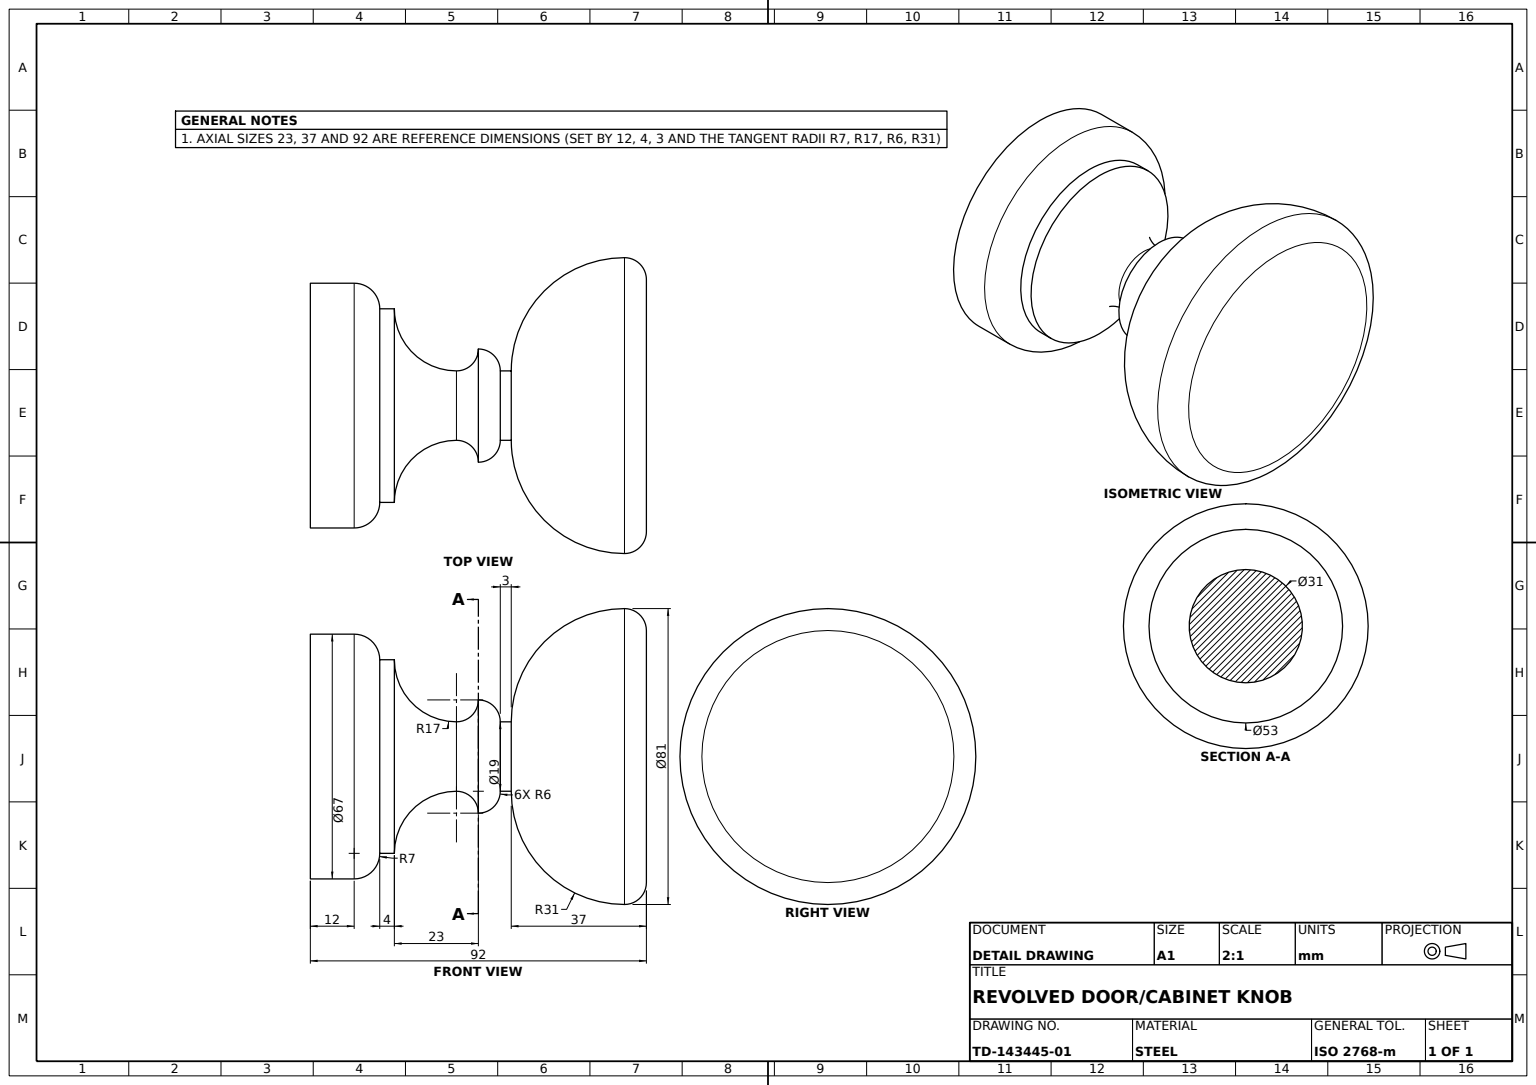
SolidWorks part; units mm, degrees
material "Plain Carbon Steel"
ref_plane "Front Plane" through (0, 0, 0) normal (0, 0, 1) x (1, 0, 0)
ref_plane "Top Plane" through (0, 0, 0) normal (0, 1, 0) x (1, 0, 0)
ref_plane "Right Plane" through (0, 0, 0) normal (1, 0, 0) x (0, 0, -1)
sketch "Knob Profile Sketch" plane through (0, 0, 0) normal (0, 0, 1) x (1, 0, 0)
  line L0 (0, 0) -> (33.5, 0)
  line L1 (33.5, 0) -> (33.5, 12)
  line L2 (26.5, 19) -> (26.5, 23)
  line L4 (0, 92) -> (0, 0)
  line L5 (9.5, 52) -> (9.5, 55)
  line L7 (34.5, 92) -> (0, 92)
  arc A0 (33.5, 12) -> (26.5, 19) centre (26.5, 12) ccw
  arc A1 (26.5, 23) -> (9.5, 40) centre (26.5, 40) cw
  arc A2 (9.5, 40) -> (15.5, 46) centre (15.5, 40) cw
  arc A3 (9.5, 52) -> (15.5, 46) centre (9.5, 46) cw
  arc A4 (9.5, 55) -> (40.5, 86) centre (9.5, 86) ccw
  arc A5 (40.5, 86) -> (34.5, 92) centre (34.5, 86) ccw
  dimension "D6" = 17
  dimension "D7" = 6
  dimension "D8" = 6
  dimension "D11" = 6
  dimension "D13" = 6
  dimension "D15" = 31
  dimension "D1" = 12
  dimension "D2" = 7
  dimension "D3" = 4
  dimension "D4" = 26.5
  dimension "D5" = 33.5
  dimension "D9" = 23
  dimension "D10" = 9.5
  dimension "D12" = 3
  dimension "D14" = 37
revolve "Knob Body Revolve" add sketch "Knob Profile Sketch" angle 360 about L4
